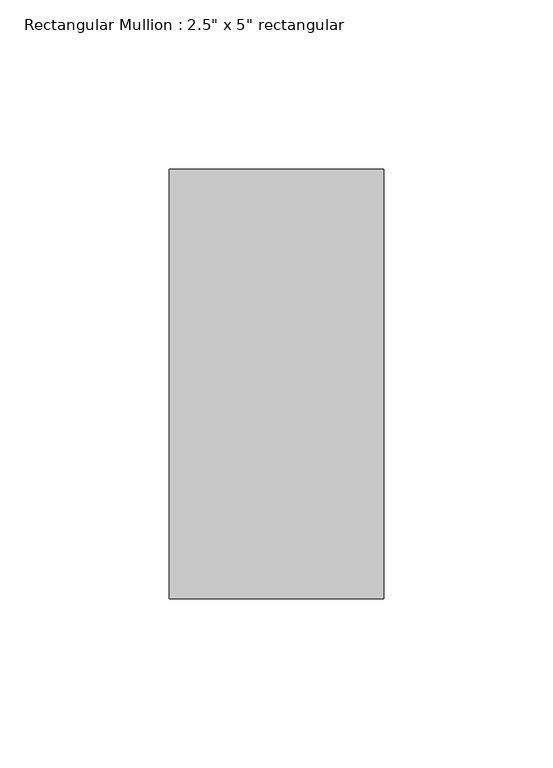
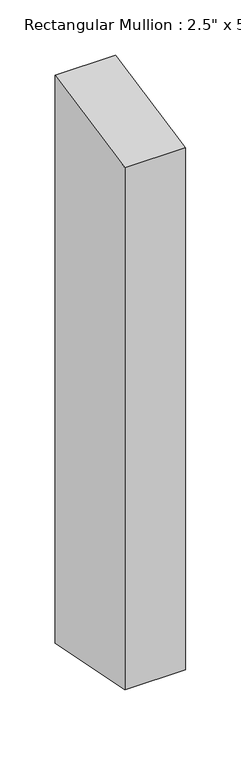
"""IFC4 building model written with IfcOpenShell, lengths in millimetres: member geometry."""

from ifc_helpers import new_model, si_unit, frame, origin, place, context, project, spatial, polyline, outline, extrude, source, transform, mapped, element, save


def member_4ff03cd1(model_context):
    return source(origin(), model_context, "Body", "SweptSolid", [
        extrude(outline(polyline([(-63.5, -12.6309353), (63.5, 12.6309353), (63.5, -615.5583104), (-63.5, -590.2964398), (-63.5, -12.6309353)])), frame((-63.5, 0.0, 0.0), z_axis=(1.0, 0.0, 0.0), x_axis=(0.0, 1.0, 0.0)), (0.0, 0.0, 1.0), 63.5),
    ])


if __name__ == "__main__":
    model = new_model("IFC4")
    model_context = context("Model", 3, world=origin())
    ifc_project = project(units=[si_unit("LENGTHUNIT", "METRE", prefix="MILLI")], contexts=[model_context])
    site = spatial("IfcSite", under=ifc_project)
    building = spatial("IfcBuilding", under=site)
    placement = place(None, origin())
    member_shape = member_4ff03cd1(model_context)
    element("IfcMember", 1, ObjectType="Rectangular Mullion : 2.5\" x 5\" rectangular", at=placement, inside=building, context=model_context, shape_type="MappedRepresentation", body=[
        mapped(member_shape, transform((0.0, 0.0, 0.0), x_axis=(1.0, 0.0, 0.0), y_axis=(0.0, 1.0, 0.0), z_axis=(0.0, 0.0, 1.0))),
    ])
    save(model, "model.ifc")

# Revit data of these elements
# Type "Rectangular Mullion : 2.5\" x 5\" rectangular"
#   built-in parameter 1007304 = 0.416667 (stored number, unit not read)
#   built-in parameter 1007301 = 0.104167 (stored number, unit not read)
#   built-in parameter 1007300 = 0.104167 (stored number, unit not read)
# Element 1 (IfcMember, "Rectangular Mullion : 2.5\" x 5\" rectangular")
#   Materials on its faces: "Iron, Ductile"
# Materials
#   "Iron, Ductile": class "Metal", colour RGB 0 0 0, transparency 0, Description = "Ductile cast iron", Cost = 0
